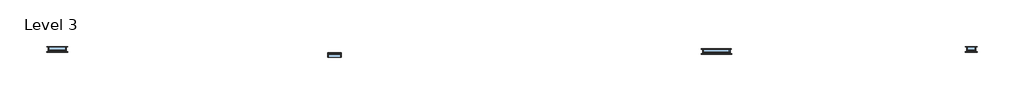
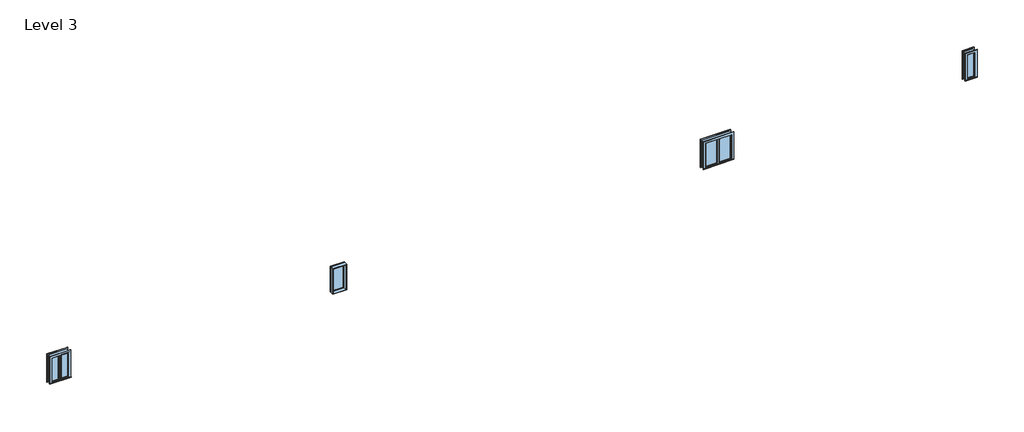
# One storey: 4 windows.
"""IFC4 building model written with IfcOpenShell, lengths in millimetres."""

from ifc_helpers import new_model, si_unit, origin, place, context, project, spatial, transform, mapped, element, save
from components import window_a765b88f, window_bb17773d, window_0862ab64, window_80bd9af0

model = new_model("IFC4")

# Units and contexts
model_context = context("Model", 3, world=origin())
ifc_project = project(units=[si_unit("LENGTHUNIT", "METRE", prefix="MILLI")], contexts=[model_context])

# Site, building, storey
site = spatial("IfcSite", under=ifc_project)
building = spatial("IfcBuilding", under=site)
storey = spatial("IfcBuildingStorey", under=building, Name="Level 3", Elevation=6096.0)

# Windows
placement = place(None, origin())
window_shape = window_a765b88f(model_context)
element("IfcWindow", 1, ObjectType="Awning with Trim : 16\" x 48\"", at=placement, inside=storey, context=model_context, shape_type="MappedRepresentation", body=[
    mapped(window_shape, transform((21730.614721, -12354.7237084, 6096.0), x_axis=(-1.0, 0.0, 0.0), y_axis=(0.0, -1.0, 0.0), z_axis=(0.0, 0.0, 1.0))),
])
window_2_shape = window_bb17773d(model_context)
element("IfcWindow", 2, ObjectType="Casement Dbl with Trim : 32\" x 48\"", at=placement, inside=storey, context=model_context, shape_type="MappedRepresentation", body=[
    mapped(window_2_shape, transform((-18960.185279, -12335.6737084, 6096.0), x_axis=(-1.0, 0.0, 0.0), y_axis=(0.0, -1.0, 0.0), z_axis=(0.0, 0.0, 1.0))),
])
window_3_shape = window_0862ab64(model_context)
element("IfcWindow", 3, ObjectType="Casement Dbl with Trim : 48\" x 48\"", at=placement, inside=storey, context=model_context, shape_type="MappedRepresentation", body=[
    mapped(window_3_shape, transform((10381.5594464, -12437.2737084, 6096.0), x_axis=(-1.0, 0.0, 0.0), y_axis=(0.0, -1.0, 0.0), z_axis=(0.0, 0.0, 1.0))),
])
window_4_shape = window_80bd9af0(model_context)
element("IfcWindow", 4, ObjectType="Fixed : 24\" x 48\"", at=placement, inside=storey, context=model_context, shape_type="MappedRepresentation", body=[
    mapped(window_4_shape, transform((-6577.685279, -12617.2007309, 6096.0), x_axis=(1.0, 0.0, 0.0), y_axis=(0.0, 1.0, 0.0), z_axis=(0.0, 0.0, 1.0))),
])

save(model, "model.ifc")

# Revit data of these elements
# Type "Awning with Trim : 16\" x 48\""
#   Type Mark = "14"
#   Construction Type Id = "GSP4R"
#   Assembly Code = "B2020100"
#   Analytic Construction = "1/8 in Pilkington single glazing"
#   Visual Light Transmittance = 0.9
#   Solar Heat Gain Coefficient = 0.78
#   Heat Transfer Coefficient (U) = 0.6496 BTU/(h·ft²·°F)
#   Height = 4' - 0"
#   Default Sill Height = 3' - 0"
#   Trim Projection - Ext. = 0' - 0 1/2"
#   Trim Projection - Int. = 0' - 0 3/4"
#   Trim Width - Exterior = 0' - 3 1/2"
#   Trim Width - Interior = 0' - 3 1/2"
#   Width = 1' - 4"
#   Window Inset = 0' - 0 3/4"
#   Define Thermal Properties by = 1
#   Glass Pane Material = Glass
#   Sash Material = Sash
#   Trim Exterior Material = Trim
#   Trim Interior Material = Trim
#   Wall Closure = (empty or 0)
# Type "Casement Dbl with Trim : 32\" x 48\""
#   Type Mark = "36"
#   Construction Type Id = "GSP4R"
#   Assembly Code = "B2020100"
#   Analytic Construction = "1/8 in Pilkington single glazing"
#   Visual Light Transmittance = 0.9
#   Solar Heat Gain Coefficient = 0.78
#   Heat Transfer Coefficient (U) = 0.6496 BTU/(h·ft²·°F)
#   Height = 4' - 0"
#   Default Sill Height = 3' - 0"
#   Trim Projection - Ext. = 0' - 0 1/2"
#   Trim Projection - Int. = 0' - 0 3/4"
#   Trim Width - Exterior = 0' - 3 1/2"
#   Trim Width - Interior = 0' - 3 1/2"
#   Width = 2' - 8"
#   Window Inset = 0' - 0 3/4"
#   Define Thermal Properties by = 1
#   Glass Pane Material = Glass
#   Sash Material = Sash
#   Trim Exterior Material = Trim
#   Trim Interior Material = Trim
#   Wall Closure = (empty or 0)
# Type "Casement Dbl with Trim : 48\" x 48\""
#   Type Mark = "34"
#   Construction Type Id = "GSP4R"
#   Assembly Code = "B2020100"
#   Analytic Construction = "1/8 in Pilkington single glazing"
#   Visual Light Transmittance = 0.9
#   Solar Heat Gain Coefficient = 0.78
#   Heat Transfer Coefficient (U) = 0.6496 BTU/(h·ft²·°F)
#   Height = 4' - 0"
#   Default Sill Height = 3' - 0"
#   Trim Projection - Ext. = 0' - 0 1/2"
#   Trim Projection - Int. = 0' - 0 3/4"
#   Trim Width - Exterior = 0' - 3 1/2"
#   Trim Width - Interior = 0' - 3 1/2"
#   Width = 4' - 0"
#   Window Inset = 0' - 0 3/4"
#   Define Thermal Properties by = 1
#   Glass Pane Material = Glass
#   Sash Material = Sash
#   Trim Exterior Material = Trim
#   Trim Interior Material = Trim
#   Wall Closure = (empty or 0)
# Type "Fixed : 24\" x 48\""
#   Type Mark = "2"
#   Construction Type Id = "GSP4R"
#   Assembly Code = "B2020100"
#   Analytic Construction = "1/8 in Pilkington single glazing"
#   Visual Light Transmittance = 0.9
#   Solar Heat Gain Coefficient = 0.78
#   Heat Transfer Coefficient (U) = 0.6496 BTU/(h·ft²·°F)
#   Height = 4' - 0"
#   Default Sill Height = 3' - 0"
#   Width = 2' - 0"
#   Window Inset = 0' - 0 3/4"
#   Define Thermal Properties by = 1
#   Glass Pane Material = Glass
#   Sash Material = Sash
#   Wall Closure = (empty or 0)
# Element 1 (IfcWindow, "Awning with Trim : 16\" x 48\"")
#   Mark = "66"
#   Phase Created = New Construction
#   Materials on its faces: "Sash", "Trim", "Glass"
# Element 2 (IfcWindow, "Casement Dbl with Trim : 32\" x 48\"")
#   Mark = "49"
#   Phase Created = New Construction
#   Materials on its faces: "Sash", "Trim", "Glass"
# Element 3 (IfcWindow, "Casement Dbl with Trim : 48\" x 48\"")
#   Mark = "15"
#   Phase Created = New Construction
#   Materials on its faces: "Sash", "Trim", "Glass"
# Element 4 (IfcWindow, "Fixed : 24\" x 48\"")
#   Mark = "83"
#   Phase Created = New Construction
#   Materials on its faces: "Sash", "Glass"
# Materials
#   "Glass": class "Glass", colour RGB 0 128 192, transparency 0.75, Description = "Soda Lime Glass", Cost = 0
#   "Sash": class "Wood", colour RGB 224 178 126, transparency 0
#   "Trim": class "Wood", colour RGB 224 178 126, transparency 0
